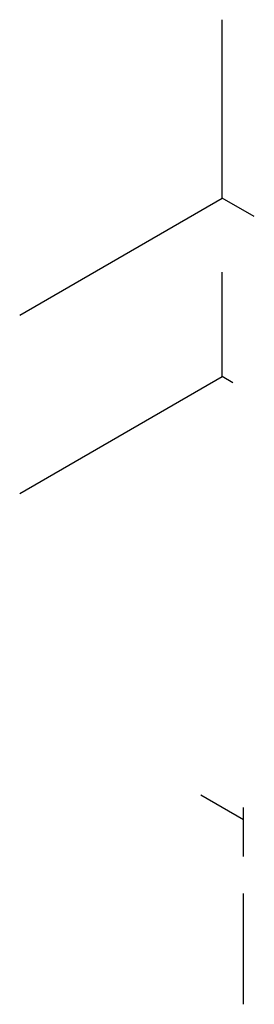
# Model space of a CAD drawing. Units: inches. Extents: x 5998 to 184806, y -27616 to 6737.
# Tile 2 of 3: x 153681 to 158520, y -13583 to 6737. Entities that reach past the tile are written whole.
import ezdxf

# ---------------------------------------------------------------- set-up
doc = ezdxf.new("R2010")
doc.units = ezdxf.units.IN
doc.header["$MEASUREMENT"] = 0
doc.layers.add('A-FURN', color=7, linetype='Continuous', lineweight=25)

msp = doc.modelspace()

# ---------------------------------------------------------------- linework, layer by layer
at = {"layer": 'A-FURN'}
for p, q in [((157860, 3054), (157860, 6737)), ((153681, 641), (157860, 3054)), ((158520, 2673), (157860, 3054)), ((157860, -629), (157860, 1530)), ((153681, -3042), (157860, -629)), ((158080, -756), (157860, -629)), ((158300, -9773), (157420, -9265)), ((158300, -10535), (158300, -9519)), ((158300, -13583), (158300, -11297))]:
    msp.add_line(p, q, dxfattribs=at)

doc.saveas('drawing.dxf')
